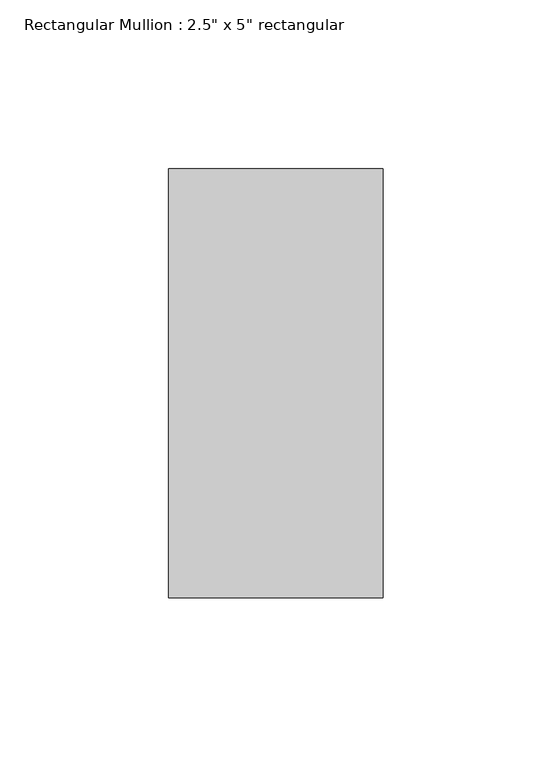
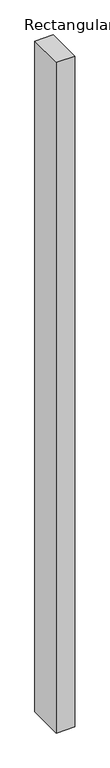
"""IFC4 building model written with IfcOpenShell, lengths in millimetres: member geometry."""

from ifc_helpers import new_model, si_unit, frame, origin, place, context, project, spatial, polyline, outline, extrude, source, transform, mapped, element, save


def member_ee409385(model_context):
    return source(origin(), model_context, "Body", "SweptSolid", [
        extrude(outline(polyline([(0.0, 63.5), (0.0, -63.5), (-63.5, -63.5), (-63.5, 63.5), (0.0, 63.5)])), frame((0.0, 0.0, -2438.4), z_axis=(0.0, 0.0, 1.0), x_axis=(1.0, 0.0, 0.0)), (0.0, 0.0, 1.0), 2438.4),
    ])


if __name__ == "__main__":
    model = new_model("IFC4")
    model_context = context("Model", 3, world=origin())
    ifc_project = project(units=[si_unit("LENGTHUNIT", "METRE", prefix="MILLI")], contexts=[model_context])
    site = spatial("IfcSite", under=ifc_project)
    building = spatial("IfcBuilding", under=site)
    placement = place(None, origin())
    member_shape = member_ee409385(model_context)
    element("IfcMember", 1, ObjectType="Rectangular Mullion : 2.5\" x 5\" rectangular", at=placement, inside=building, context=model_context, shape_type="MappedRepresentation", body=[
        mapped(member_shape, transform((0.0, 0.0, 0.0), x_axis=(1.0, 0.0, 0.0), y_axis=(0.0, 1.0, 0.0), z_axis=(0.0, 0.0, 1.0))),
    ])
    save(model, "model.ifc")

# Revit data of these elements
# Type "Rectangular Mullion : 2.5\" x 5\" rectangular"
#   built-in parameter 1007304 = 0.416667 (stored number, unit not read)
#   built-in parameter 1007301 = 0.104167 (stored number, unit not read)
#   built-in parameter 1007300 = 0.104167 (stored number, unit not read)
# Element 1 (IfcMember, "Rectangular Mullion : 2.5\" x 5\" rectangular")
#   Materials on its faces: "Aluminum"
# Materials
#   "Aluminum": class "Metal", colour RGB 247 247 247, transparency 0, Description = "Aluminum 6061", Cost = 0
